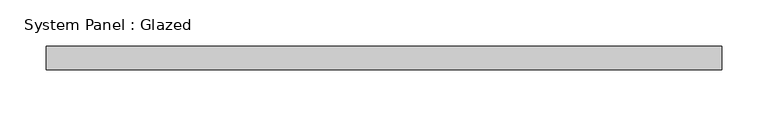
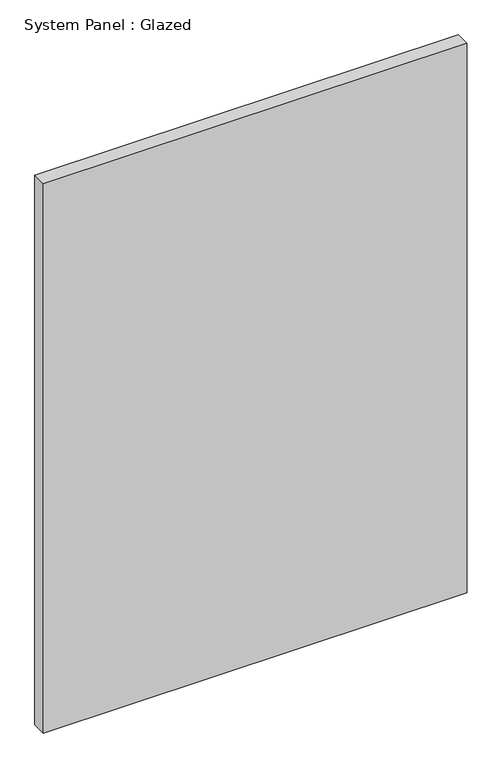
"""IFC4 building model written with IfcOpenShell, lengths in millimetres: plate geometry, System Panel : Glazed."""

from ifc_helpers import new_model, si_unit, origin, origin_with_axes, place, context, project, spatial, polyline, outline, extrude, source, transform, mapped, element, save


def system_panel_glazed_c5f71645(model_context):
    return source(origin(), model_context, "Body", "SweptSolid", [
        extrude(outline(polyline([(366.1833333, 19.05), (-366.1833333, 19.05), (-366.1833333, 44.45), (366.1833333, 44.45), (366.1833333, 19.05)])), origin_with_axes(), (0.0, 0.0, 1.0), 1003.3),
    ])


if __name__ == "__main__":
    model = new_model("IFC4")
    model_context = context("Model", 3, world=origin())
    ifc_project = project(units=[si_unit("LENGTHUNIT", "METRE", prefix="MILLI")], contexts=[model_context])
    site = spatial("IfcSite", under=ifc_project)
    building = spatial("IfcBuilding", under=site)
    placement = place(None, origin())
    system_panel_glazed_shape = system_panel_glazed_c5f71645(model_context)
    element("IfcPlate", 1, ObjectType="System Panel : Glazed", at=placement, inside=building, context=model_context, shape_type="MappedRepresentation", body=[
        mapped(system_panel_glazed_shape, transform((0.0, 0.0, 0.0), x_axis=(1.0, 0.0, 0.0), y_axis=(0.0, 1.0, 0.0), z_axis=(0.0, 0.0, 1.0))),
    ])
    save(model, "model.ifc")

# Revit data of these elements
# Type "System Panel : Glazed"
#   Construction Type Id = "GSP4R"
#   Analytic Construction = "1/8 in Pilkington single glazing"
#   Visual Light Transmittance = 0.9
#   Solar Heat Gain Coefficient = 0.86
#   Heat Transfer Coefficient (U) = 1.18115 BTU/(h·ft²·°F)
# Element 1 (IfcPlate, "System Panel : Glazed")
#   Materials on its faces: "Glass"
# Materials
#   "Glass": class "Glass", colour RGB 0 128 192, transparency 0.75, Description = "Soda Lime Glass", Cost = 0
